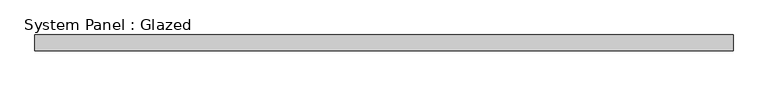
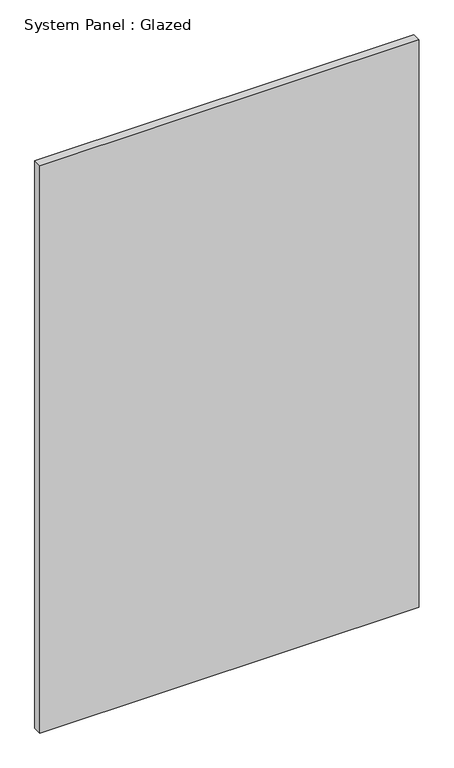
"""IFC4 building model written with IfcOpenShell, lengths in millimetres: plate geometry, System Panel : Glazed."""

from ifc_helpers import new_model, si_unit, origin, origin_with_axes, place, context, project, spatial, polyline, outline, extrude, source, transform, mapped, element, save


def system_panel_glazed_71021e01(model_context):
    return source(origin(), model_context, "Body", "SweptSolid", [
        extrude(outline(polyline([(546.5, 24.5), (-546.5, 24.5), (-546.5, 49.5), (546.5, 49.5), (546.5, 24.5)])), origin_with_axes(), (0.0, 0.0, 1.0), 1728.8),
    ])


if __name__ == "__main__":
    model = new_model("IFC4")
    model_context = context("Model", 3, world=origin())
    ifc_project = project(units=[si_unit("LENGTHUNIT", "METRE", prefix="MILLI")], contexts=[model_context])
    site = spatial("IfcSite", under=ifc_project)
    building = spatial("IfcBuilding", under=site)
    placement = place(None, origin())
    system_panel_glazed_shape = system_panel_glazed_71021e01(model_context)
    element("IfcPlate", 1, ObjectType="System Panel : Glazed", at=placement, inside=building, context=model_context, shape_type="MappedRepresentation", body=[
        mapped(system_panel_glazed_shape, transform((0.0, 0.0, 0.0), x_axis=(1.0, 0.0, 0.0), y_axis=(0.0, 1.0, 0.0), z_axis=(0.0, 0.0, 1.0))),
    ])
    save(model, "model.ifc")

# Revit data of these elements
# Type "System Panel : Glazed"
#   Construction Type Id = "GSP4R"
#   Analytic Construction = "1/8 in Pilkington single glazing"
#   Visual Light Transmittance = 0.9
#   Solar Heat Gain Coefficient = 0.86
#   Heat Transfer Coefficient (U) = 6.7069 W/(m²·K)
# Element 1 (IfcPlate, "System Panel : Glazed")
#   Materials on its faces: "Glass"
# Materials
#   "Glass": class "Glass", colour RGB 0 128 192, transparency 0.9, Description = "Soda Lime Glass", Cost = 0
